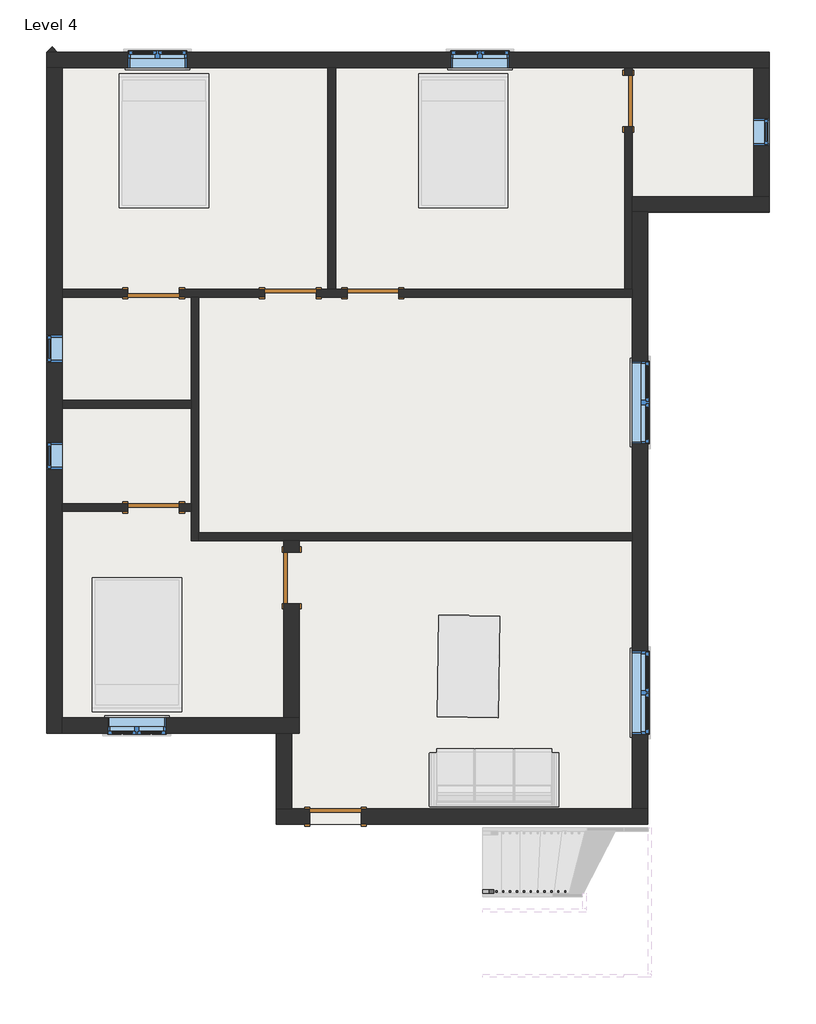
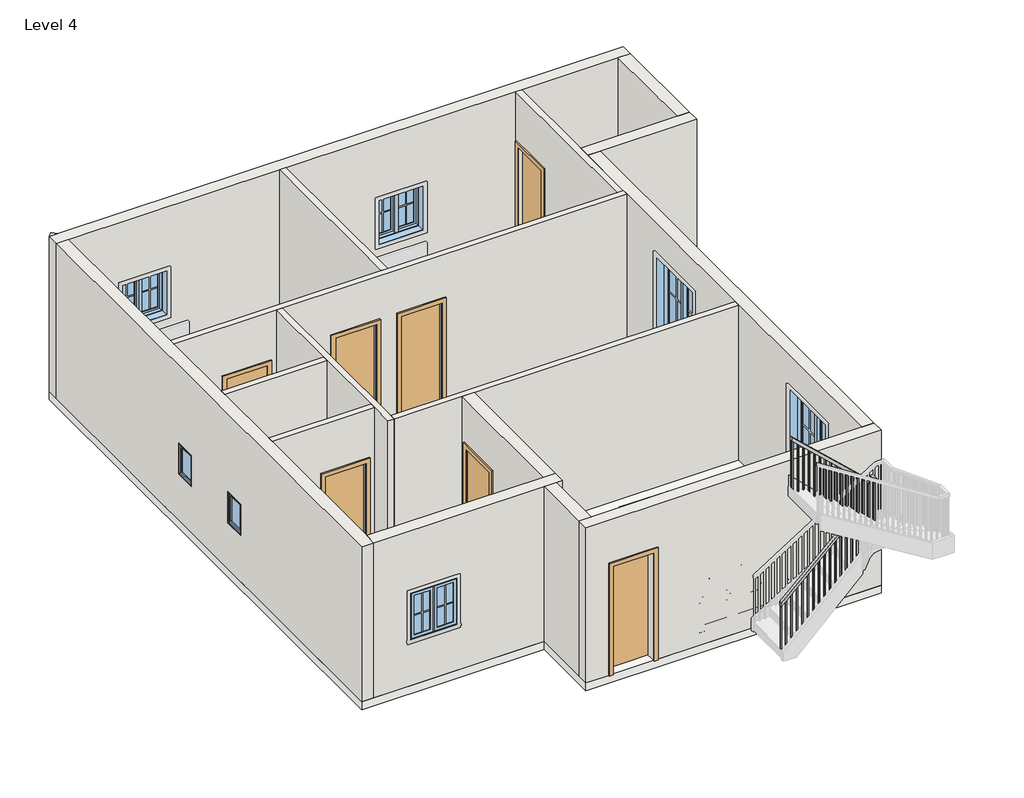
# One storey, part 1 of 2: 17 walls, 8 windows, 7 doors, 1 railing, 1 roof.
"""IFC4 building model written with IfcOpenShell, lengths in millimetres."""

from ifc_helpers import new_model, si_unit, frame, origin, place, context, project, spatial, polyline, outline, extrude, faceted_brep, transform, mapped, element, save
from components import door_f2b275c1, door_d8f5dbb5, door_214872d5, door_78caadf7, door_bb98abfd, window_aa618e30, window_339605e1, window_8377141f

model = new_model("IFC4")

# Units and contexts
model_context = context("Model", 3, world=origin())
ifc_project = project(units=[si_unit("LENGTHUNIT", "METRE", prefix="MILLI")], contexts=[model_context])

# Site, building, storey
site = spatial("IfcSite", under=ifc_project)
building = spatial("IfcBuilding", under=site)
storey = spatial("IfcBuildingStorey", under=building, Name="Level 4", Elevation=6400.8)

# Doors
placement = place(None, origin())
door_shape = door_f2b275c1(model_context)
element("IfcDoor", 1, ObjectType="Single-Flush : 30\" x 80\"", at=placement, inside=storey, context=model_context, shape_type="MappedRepresentation", body=[
    mapped(door_shape, transform((2459.5084916, 7319.9935985, 6400.8), x_axis=(0.0, 1.0, 0.0), y_axis=(-1.0, 0.0, 0.0), z_axis=(0.0, 0.0, 1.0))),
])
element("IfcDoor", 2, ObjectType="Single-Flush : 30\" x 80\"", at=placement, inside=storey, context=model_context, shape_type="MappedRepresentation", body=[
    mapped(door_shape, transform((-4550.8915084, 4481.5435985, 6400.8), x_axis=(1.0, 0.0, 0.0), y_axis=(0.0, 1.0, 0.0), z_axis=(0.0, 0.0, 1.0))),
])
door_2_shape = door_d8f5dbb5(model_context)
element("IfcDoor", 3, ObjectType="Single-Flush : 30\" x 80\"", at=placement, inside=storey, context=model_context, shape_type="MappedRepresentation", body=[
    mapped(door_2_shape, transform((-4550.8915084, 1319.2435985, 6400.8), x_axis=(1.0, 0.0, 0.0), y_axis=(0.0, 1.0, 0.0), z_axis=(0.0, 0.0, 1.0))),
])
door_3_shape = door_214872d5(model_context)
element("IfcDoor", 4, ObjectType="Single-Flush : 30\" x 84\"", at=placement, inside=storey, context=model_context, shape_type="MappedRepresentation", body=[
    mapped(door_3_shape, transform((-2531.5915084, 4481.5435985, 6400.8), x_axis=(1.0, 0.0, 0.0), y_axis=(0.0, 1.0, 0.0), z_axis=(0.0, 0.0, 1.0))),
])
door_4_shape = door_78caadf7(model_context)
element("IfcDoor", 5, ObjectType="Single-Flush : 30\" x 84\"", at=placement, inside=storey, context=model_context, shape_type="MappedRepresentation", body=[
    mapped(door_4_shape, transform((-1312.3915084, 4481.5435985, 6400.8), x_axis=(-1.0, 0.0, 0.0), y_axis=(0.0, -1.0, 0.0), z_axis=(0.0, 0.0, 1.0))),
])
door_5_shape = door_bb98abfd(model_context)
element("IfcDoor", 6, ObjectType="Single-Flush : 30\" x 84\"", at=placement, inside=storey, context=model_context, shape_type="MappedRepresentation", body=[
    mapped(door_5_shape, transform((-2512.5415084, 277.8435985, 6400.8), x_axis=(0.0, 1.0, 0.0), y_axis=(-1.0, 0.0, 0.0), z_axis=(0.0, 0.0, 1.0))),
])
element("IfcDoor", 7, ObjectType="Single-Flush : 30\" x 84\"", at=placement, inside=storey, context=model_context, shape_type="MappedRepresentation", body=[
    mapped(door_5_shape, transform((-1864.8415084, -3246.4064015, 6400.8), x_axis=(1.0, 0.0, 0.0), y_axis=(0.0, 1.0, 0.0), z_axis=(0.0, 0.0, 1.0))),
])

# Railing
element("IfcRailing", 8, ObjectType="Handrail - Rectangular", at=placement, inside=storey, context=model_context, shape_type="SolidModel", body=[
    faceted_brep([(306.9570026, -4325.9064015, 7518.4), (306.9570026, -4325.9064015, 7448.9424448), (306.9570026, -4376.7064015, 7448.9424448), (306.9570026, -4376.7064015, 7518.4), (1758.4886944, -4325.9064015, 8871.8629243), (1809.2886944, -4325.9064015, 8849.773206), (1809.2886944, -4376.7064015, 8849.773206), (1758.4886944, -4376.7064015, 8871.8629243), (1758.4886944, -4325.9064015, 9115.4738258), (1809.2886944, -4325.9064015, 9064.6738258), (1809.2886944, -4376.7064015, 9064.6738258), (1758.4886944, -4376.7064015, 9115.4738258), (1885.4886944, -4325.9064015, 9115.4738258), (1885.4886944, -4325.9064015, 9064.6738258), (1834.6886944, -4376.7064015, 9064.6738258), (1834.6886944, -4376.7064015, 9115.4738258), (1885.4886944, -4452.9064015, 9115.4738258), (1885.4886944, -4484.6424812, 9064.6738258), (1834.6886944, -4484.6424812, 9064.6738258), (1834.6886944, -4452.9064015, 9115.4738258), (1885.4886944, -4579.9064015, 9375.7261742), (1885.4886944, -4630.7064015, 9363.9925523), (1834.6886944, -4630.7064015, 9363.9925523), (1834.6886944, -4579.9064015, 9375.7261742), (1885.4886944, -4579.9064015, 9619.3370757), (1885.4886944, -4630.7064015, 9568.5370757), (1834.6886944, -4630.7064015, 9568.5370757), (1834.6886944, -4579.9064015, 9619.3370757), (1885.4886944, -4706.9064015, 9619.3370757), (1885.4886944, -4706.9064015, 9568.5370757), (1834.6886944, -4656.1064015, 9568.5370757), (1834.6886944, -4656.1064015, 9619.3370757), (1758.4886944, -4706.9064015, 9619.3370757), (1738.4792562, -4706.9064015, 9568.5370757), (1738.4792562, -4656.1064015, 9568.5370757), (1758.4886944, -4656.1064015, 9619.3370757), (306.9570026, -4706.9064015, 10972.8), (306.9570026, -4656.1064015, 10972.8), (306.9570026, -4656.1064015, 10903.3424448), (306.9570026, -4706.9064015, 10903.3424448)], [[[0, 1, 2, 3]], [[1, 0, 4, 5]], [[2, 1, 5, 6]], [[3, 2, 6, 7]], [[0, 3, 7, 4]], [[5, 4, 8, 9]], [[6, 5, 9, 10]], [[7, 6, 10, 11]], [[4, 7, 11, 8]], [[9, 8, 12, 13]], [[10, 9, 13, 14]], [[11, 10, 14, 15]], [[8, 11, 15, 12]], [[13, 12, 16, 17]], [[14, 13, 17, 18]], [[15, 14, 18, 19]], [[12, 15, 19, 16]], [[17, 16, 20, 21]], [[18, 17, 21, 22]], [[19, 18, 22, 23]], [[16, 19, 23, 20]], [[21, 20, 24, 25]], [[22, 21, 25, 26]], [[23, 22, 26, 27]], [[20, 23, 27, 24]], [[25, 24, 28, 29]], [[26, 25, 29, 30]], [[27, 26, 30, 31]], [[24, 27, 31, 28]], [[29, 28, 32, 33]], [[30, 29, 33, 34]], [[31, 30, 34, 35]], [[28, 31, 35, 32]], [[36, 37, 38, 39]], [[33, 32, 36, 39]], [[34, 33, 39, 38]], [[35, 34, 38, 37]], [[32, 35, 37, 36]]]),
    extrude(outline(polyline([(10867.2974865, 345.6136944), (10885.0604254, 326.5636944), (9855.2, 326.5636944), (9855.2, 345.6136944), (10867.2974865, 345.6136944)])), frame((0.0, -4691.0314015, 0.0), z_axis=(0.0, 1.0, 0.0), x_axis=(0.0, 0.0, 1.0)), (0.0, 0.0, 1.0), 19.05),
    extrude(outline(polyline([(10772.5618126, 447.2136944), (10790.3247514, 428.1636944), (9855.2, 428.1636944), (9855.2, 447.2136944), (10772.5618126, 447.2136944)])), frame((0.0, -4691.0314015, 0.0), z_axis=(0.0, 1.0, 0.0), x_axis=(0.0, 0.0, 1.0)), (0.0, 0.0, 1.0), 19.05),
    extrude(outline(polyline([(10677.8261386, 548.8136944), (10695.5890775, 529.7636944), (9855.2, 529.7636944), (9855.2, 548.8136944), (10677.8261386, 548.8136944)])), frame((0.0, -4691.0314015, 0.0), z_axis=(0.0, 1.0, 0.0), x_axis=(0.0, 0.0, 1.0)), (0.0, 0.0, 1.0), 19.05),
    extrude(outline(polyline([(10583.0904646, 650.4136944), (10600.8534035, 631.3636944), (9652.0, 631.3636944), (9652.0, 650.4136944), (10583.0904646, 650.4136944)])), frame((0.0, -4691.0314015, 0.0), z_axis=(0.0, 1.0, 0.0), x_axis=(0.0, 0.0, 1.0)), (0.0, 0.0, 1.0), 19.05),
    extrude(outline(polyline([(10488.3547907, 752.0136944), (10506.1177295, 732.9636944), (9652.0, 732.9636944), (9652.0, 752.0136944), (10488.3547907, 752.0136944)])), frame((0.0, -4691.0314015, 0.0), z_axis=(0.0, 1.0, 0.0), x_axis=(0.0, 0.0, 1.0)), (0.0, 0.0, 1.0), 19.05),
    extrude(outline(polyline([(10393.6191167, 853.6136944), (10411.3820556, 834.5636944), (9652.0, 834.5636944), (9652.0, 853.6136944), (10393.6191167, 853.6136944)])), frame((0.0, -4691.0314015, 0.0), z_axis=(0.0, 1.0, 0.0), x_axis=(0.0, 0.0, 1.0)), (0.0, 0.0, 1.0), 19.05),
    extrude(outline(polyline([(10298.8834427, 955.2136944), (10316.6463816, 936.1636944), (9448.8, 936.1636944), (9448.8, 955.2136944), (10298.8834427, 955.2136944)])), frame((0.0, -4691.0314015, 0.0), z_axis=(0.0, 1.0, 0.0), x_axis=(0.0, 0.0, 1.0)), (0.0, 0.0, 1.0), 19.05),
    extrude(outline(polyline([(10204.1477688, 1056.8136944), (10221.9107076, 1037.7636944), (9448.8, 1037.7636944), (9448.8, 1056.8136944), (10204.1477688, 1056.8136944)])), frame((0.0, -4691.0314015, 0.0), z_axis=(0.0, 1.0, 0.0), x_axis=(0.0, 0.0, 1.0)), (0.0, 0.0, 1.0), 19.05),
    extrude(outline(polyline([(10109.4120948, 1158.4136944), (10127.1750337, 1139.3636944), (9245.6, 1139.3636944), (9245.6, 1158.4136944), (10109.4120948, 1158.4136944)])), frame((0.0, -4691.0314015, 0.0), z_axis=(0.0, 1.0, 0.0), x_axis=(0.0, 0.0, 1.0)), (0.0, 0.0, 1.0), 19.05),
    extrude(outline(polyline([(10014.6764208, 1260.0136944), (10032.4393597, 1240.9636944), (9245.6, 1240.9636944), (9245.6, 1260.0136944), (10014.6764208, 1260.0136944)])), frame((0.0, -4691.0314015, 0.0), z_axis=(0.0, 1.0, 0.0), x_axis=(0.0, 0.0, 1.0)), (0.0, 0.0, 1.0), 19.05),
    extrude(outline(polyline([(9919.9407469, 1361.6136944), (9937.7036857, 1342.5636944), (9245.6, 1342.5636944), (9245.6, 1361.6136944), (9919.9407469, 1361.6136944)])), frame((0.0, -4691.0314015, 0.0), z_axis=(0.0, 1.0, 0.0), x_axis=(0.0, 0.0, 1.0)), (0.0, 0.0, 1.0), 19.05),
    extrude(outline(polyline([(9825.2050729, 1463.2136944), (9842.9680118, 1444.1636944), (9042.4, 1444.1636944), (9042.4, 1463.2136944), (9825.2050729, 1463.2136944)])), frame((0.0, -4691.0314015, 0.0), z_axis=(0.0, 1.0, 0.0), x_axis=(0.0, 0.0, 1.0)), (0.0, 0.0, 1.0), 19.05),
    extrude(outline(polyline([(9730.4693989, 1564.8136944), (9748.2323378, 1545.7636944), (9042.4, 1545.7636944), (9042.4, 1564.8136944), (9730.4693989, 1564.8136944)])), frame((0.0, -4691.0314015, 0.0), z_axis=(0.0, 1.0, 0.0), x_axis=(0.0, 0.0, 1.0)), (0.0, 0.0, 1.0), 19.05),
    extrude(outline(polyline([(9635.733725, 1666.4136944), (9653.4966638, 1647.3636944), (8839.2, 1647.3636944), (8839.2, 1666.4136944), (9635.733725, 1666.4136944)])), frame((0.0, -4691.0314015, 0.0), z_axis=(0.0, 1.0, 0.0), x_axis=(0.0, 0.0, 1.0)), (0.0, 0.0, 1.0), 19.05),
    extrude(outline(polyline([(9540.998051, 1768.0136944), (9558.7609899, 1748.9636944), (8839.2, 1748.9636944), (8839.2, 1768.0136944), (9540.998051, 1768.0136944)])), frame((0.0, -4691.0314015, 0.0), z_axis=(0.0, 1.0, 0.0), x_axis=(0.0, 0.0, 1.0)), (0.0, 0.0, 1.0), 19.05),
    extrude(outline(polyline([(1850.5636944, -4646.5814015), (1869.6136944, -4646.5814015), (1869.6136944, -4665.6314015), (1850.5636944, -4665.6314015), (1850.5636944, -4646.5814015)])), frame((0.0, 0.0, 8432.8), z_axis=(0.0, 0.0, 1.0), x_axis=(1.0, 0.0, 0.0)), (0.0, 0.0, 1.0), 1135.7370757),
    extrude(outline(polyline([(-4564.0314015, 9227.3600694), (-4544.9814015, 9188.3222172), (-4544.9814015, 8229.6), (-4564.0314015, 8229.6), (-4564.0314015, 9227.3600694)])), frame((1850.5636944, 0.0, 0.0), z_axis=(1.0, 0.0, 0.0), x_axis=(0.0, 1.0, 0.0)), (0.0, 0.0, 1.0), 19.05),
    extrude(outline(polyline([(-4462.4314015, 9019.1581907), (-4443.3814015, 8980.1203385), (-4443.3814015, 8026.4), (-4462.4314015, 8026.4), (-4462.4314015, 9019.1581907)])), frame((1850.5636944, 0.0, 0.0), z_axis=(1.0, 0.0, 0.0), x_axis=(0.0, 1.0, 0.0)), (0.0, 0.0, 1.0), 19.05),
    extrude(outline(polyline([(1821.4320026, -4360.8314015), (1821.4320026, -4341.7814015), (1840.4820026, -4341.7814015), (1840.4820026, -4360.8314015), (1821.4320026, -4360.8314015)])), frame((0.0, 0.0, 7823.2), z_axis=(0.0, 0.0, 1.0), x_axis=(1.0, 0.0, 0.0)), (0.0, 0.0, 1.0), 1241.4738258),
    extrude(outline(polyline([(8784.1233497, 1738.8820026), (8766.3604108, 1719.8320026), (7620.0, 1719.8320026), (7620.0, 1738.8820026), (8784.1233497, 1738.8820026)])), frame((0.0, -4360.8314015, 0.0), z_axis=(0.0, 1.0, 0.0), x_axis=(0.0, 0.0, 1.0)), (0.0, 0.0, 1.0), 19.05),
    extrude(outline(polyline([(8689.3876757, 1637.2820026), (8671.6247369, 1618.2320026), (7620.0, 1618.2320026), (7620.0, 1637.2820026), (8689.3876757, 1637.2820026)])), frame((0.0, -4360.8314015, 0.0), z_axis=(0.0, 1.0, 0.0), x_axis=(0.0, 0.0, 1.0)), (0.0, 0.0, 1.0), 19.05),
    extrude(outline(polyline([(8594.6520018, 1535.6820026), (8576.8890629, 1516.6320026), (7416.8, 1516.6320026), (7416.8, 1535.6820026), (8594.6520018, 1535.6820026)])), frame((0.0, -4360.8314015, 0.0), z_axis=(0.0, 1.0, 0.0), x_axis=(0.0, 0.0, 1.0)), (0.0, 0.0, 1.0), 19.05),
    extrude(outline(polyline([(8499.9163278, 1434.0820026), (8482.1533889, 1415.0320026), (7416.8, 1415.0320026), (7416.8, 1434.0820026), (8499.9163278, 1434.0820026)])), frame((0.0, -4360.8314015, 0.0), z_axis=(0.0, 1.0, 0.0), x_axis=(0.0, 0.0, 1.0)), (0.0, 0.0, 1.0), 19.05),
    extrude(outline(polyline([(8405.1806538, 1332.4820026), (8387.417715, 1313.4320026), (7213.6, 1313.4320026), (7213.6, 1332.4820026), (8405.1806538, 1332.4820026)])), frame((0.0, -4360.8314015, 0.0), z_axis=(0.0, 1.0, 0.0), x_axis=(0.0, 0.0, 1.0)), (0.0, 0.0, 1.0), 19.05),
    extrude(outline(polyline([(8310.4449799, 1230.8820026), (8292.682041, 1211.8320026), (7213.6, 1211.8320026), (7213.6, 1230.8820026), (8310.4449799, 1230.8820026)])), frame((0.0, -4360.8314015, 0.0), z_axis=(0.0, 1.0, 0.0), x_axis=(0.0, 0.0, 1.0)), (0.0, 0.0, 1.0), 19.05),
    extrude(outline(polyline([(8215.7093059, 1129.2820026), (8197.946367, 1110.2320026), (7010.4, 1110.2320026), (7010.4, 1129.2820026), (8215.7093059, 1129.2820026)])), frame((0.0, -4360.8314015, 0.0), z_axis=(0.0, 1.0, 0.0), x_axis=(0.0, 0.0, 1.0)), (0.0, 0.0, 1.0), 19.05),
    extrude(outline(polyline([(8120.9736319, 1027.6820026), (8103.2106931, 1008.6320026), (7010.4, 1008.6320026), (7010.4, 1027.6820026), (8120.9736319, 1027.6820026)])), frame((0.0, -4360.8314015, 0.0), z_axis=(0.0, 1.0, 0.0), x_axis=(0.0, 0.0, 1.0)), (0.0, 0.0, 1.0), 19.05),
    extrude(outline(polyline([(8026.237958, 926.0820026), (8008.4750191, 907.0320026), (7010.4, 907.0320026), (7010.4, 926.0820026), (8026.237958, 926.0820026)])), frame((0.0, -4360.8314015, 0.0), z_axis=(0.0, 1.0, 0.0), x_axis=(0.0, 0.0, 1.0)), (0.0, 0.0, 1.0), 19.05),
    extrude(outline(polyline([(7931.502284, 824.4820026), (7913.7393451, 805.4320026), (6807.2, 805.4320026), (6807.2, 824.4820026), (7931.502284, 824.4820026)])), frame((0.0, -4360.8314015, 0.0), z_axis=(0.0, 1.0, 0.0), x_axis=(0.0, 0.0, 1.0)), (0.0, 0.0, 1.0), 19.05),
    extrude(outline(polyline([(7836.7666101, 722.8820026), (7819.0036712, 703.8320026), (6807.2, 703.8320026), (6807.2, 722.8820026), (7836.7666101, 722.8820026)])), frame((0.0, -4360.8314015, 0.0), z_axis=(0.0, 1.0, 0.0), x_axis=(0.0, 0.0, 1.0)), (0.0, 0.0, 1.0), 19.05),
    extrude(outline(polyline([(7742.0309361, 621.2820026), (7724.2679972, 602.2320026), (6807.2, 602.2320026), (6807.2, 621.2820026), (7742.0309361, 621.2820026)])), frame((0.0, -4360.8314015, 0.0), z_axis=(0.0, 1.0, 0.0), x_axis=(0.0, 0.0, 1.0)), (0.0, 0.0, 1.0), 19.05),
    extrude(outline(polyline([(7647.2952621, 519.6820026), (7629.5323233, 500.6320026), (6604.0, 500.6320026), (6604.0, 519.6820026), (7647.2952621, 519.6820026)])), frame((0.0, -4360.8314015, 0.0), z_axis=(0.0, 1.0, 0.0), x_axis=(0.0, 0.0, 1.0)), (0.0, 0.0, 1.0), 19.05),
    extrude(outline(polyline([(7552.5595882, 418.0820026), (7534.7966493, 399.0320026), (6604.0, 399.0320026), (6604.0, 418.0820026), (7552.5595882, 418.0820026)])), frame((0.0, -4360.8314015, 0.0), z_axis=(0.0, 1.0, 0.0), x_axis=(0.0, 0.0, 1.0)), (0.0, 0.0, 1.0), 19.05),
    extrude(outline(polyline([(1850.5636944, -4671.9814015), (1869.6136944, -4671.9814015), (1869.6136944, -4691.0314015), (1850.5636944, -4691.0314015), (1850.5636944, -4671.9814015)])), frame((0.0, 0.0, 8636.0), z_axis=(0.0, 0.0, 1.0), x_axis=(1.0, 0.0, 0.0)), (0.0, 0.0, 1.0), 932.5370757),
    extrude(outline(polyline([(1850.5636944, -4360.8314015), (1850.5636944, -4341.7814015), (1869.6136944, -4341.7814015), (1869.6136944, -4360.8314015), (1850.5636944, -4360.8314015)])), frame((0.0, 0.0, 7823.2), z_axis=(0.0, 0.0, 1.0), x_axis=(1.0, 0.0, 0.0)), (0.0, 0.0, 1.0), 1241.4738258),
    extrude(outline(polyline([(10885.5795059, 326.0070026), (10903.3424448, 306.9570026), (9855.2, 306.9570026), (9855.2, 326.0070026), (10885.5795059, 326.0070026)])), frame((0.0, -4691.0314015, 0.0), z_axis=(0.0, 1.0, 0.0), x_axis=(0.0, 0.0, 1.0)), (0.0, 0.0, 1.0), 19.05),
    extrude(outline(polyline([(7466.7053836, 326.0070026), (7448.9424448, 306.9570026), (6604.0, 306.9570026), (6604.0, 326.0070026), (7466.7053836, 326.0070026)])), frame((0.0, -4360.8314015, 0.0), z_axis=(0.0, 1.0, 0.0), x_axis=(0.0, 0.0, 1.0)), (0.0, 0.0, 1.0), 19.05),
])

# Roof
element("IfcRoof", 9, ObjectType="Generic - 12\"", at=placement, inside=storey, context=model_context, shape_type="SweptSolid", body=[
    extrude(outline(polyline([(-6132.0415084, 8043.8940003), (4535.9584916, 8043.8940003), (4535.9584916, 5681.6935985), (2745.2584916, 5681.6935985), (2745.2584916, -3360.7064015), (-2741.1415084, -3360.7064015), (-2741.1415084, -2014.5064015), (-6132.0415084, -2014.5064015), (-6132.0415084, 8043.8940003)])), frame((0.0, 0.0, 6248.4), z_axis=(0.0, 0.0, 1.0), x_axis=(1.0, 0.0, 0.0)), (0.0, 0.0, 1.0), 152.4),
])

# Walls
element("IfcWall", 10, ObjectType="WALL4.5\"", at=placement, inside=storey, context=model_context, shape_type="SweptSolid", body=[
    extrude(outline(polyline([(-1979.1415084, 4538.6935985), (-1979.1415084, 7815.2935985), (-1864.8415084, 7815.2935985), (-1864.8415084, 4538.6935985), (-1979.1415084, 4538.6935985)])), frame((0.0, 0.0, 6400.8), z_axis=(0.0, 0.0, 1.0), x_axis=(1.0, 0.0, 0.0)), (0.0, 0.0, 1.0), 3048.0),
])
element("IfcWall", 11, ObjectType="WALL4.5\"", at=placement, inside=storey, context=model_context, shape_type="Brep", body=[
    faceted_brep([(-2150.5915084, 4424.3935985, 6400.8), (-1693.3915084, 4424.3935985, 6400.8), (-1693.3915084, 4424.3935985, 8534.4), (-931.3915084, 4424.3935985, 8534.4), (-931.3915084, 4424.3935985, 6400.8), (2516.6584916, 4424.3935985, 6400.8), (2516.6584916, 4424.3935985, 9448.8), (-3884.1415084, 4424.3935985, 9448.8), (-3998.4415084, 4424.3935985, 9448.8), (-5903.4415084, 4424.3935985, 9448.8), (-5903.4415084, 4424.3935985, 6400.8), (-4931.8915084, 4424.3935985, 6400.8), (-4931.8915084, 4424.3935985, 8432.8), (-4169.8915084, 4424.3935985, 8432.8), (-4169.8915084, 4424.3935985, 6400.8), (-3998.4415084, 4424.3935985, 6400.8), (-3884.1415084, 4424.3935985, 6400.8), (-2912.5915084, 4424.3935985, 6400.8), (-2912.5915084, 4424.3935985, 8534.4), (-2150.5915084, 4424.3935985, 8534.4), (-1693.3915084, 4538.6935985, 8534.4), (-1693.3915084, 4538.6935985, 6400.8), (-1864.8415084, 4538.6935985, 6400.8), (-1979.1415084, 4538.6935985, 6400.8), (-2150.5915084, 4538.6935985, 6400.8), (-2150.5915084, 4538.6935985, 8534.4), (-2912.5915084, 4538.6935985, 8534.4), (-2912.5915084, 4538.6935985, 6400.8), (-4169.8915084, 4538.6935985, 6400.8), (-4169.8915084, 4538.6935985, 8432.8), (-4931.8915084, 4538.6935985, 8432.8), (-4931.8915084, 4538.6935985, 6400.8), (-5903.4415084, 4538.6935985, 6400.8), (-5903.4415084, 4538.6935985, 9448.8), (-1979.1415084, 4538.6935985, 9448.8), (-1864.8415084, 4538.6935985, 9448.8), (2402.3584916, 4538.6935985, 9448.8), (2516.6584916, 4538.6935985, 9448.8), (2516.6584916, 4538.6935985, 6400.8), (2402.3584916, 4538.6935985, 6400.8), (-931.3915084, 4538.6935985, 6400.8), (-931.3915084, 4538.6935985, 8534.4)], [[[0, 1, 2, 3, 4, 5, 6, 7, 8, 9, 10, 11, 12, 13, 14, 15, 16, 17, 18, 19]], [[20, 21, 22, 23, 24, 25, 26, 27, 28, 29, 30, 31, 32, 33, 34, 35, 36, 37, 38, 39, 40, 41]], [[11, 10, 32, 31]], [[17, 16, 15, 14, 28, 27]], [[40, 39, 38, 5, 4]], [[24, 23, 22, 21, 1, 0]], [[10, 9, 33, 32]], [[6, 5, 38, 37]], [[29, 28, 14, 13]], [[30, 29, 13, 12]], [[31, 30, 12, 11]], [[25, 24, 0, 19]], [[26, 25, 19, 18]], [[27, 26, 18, 17]], [[2, 1, 21, 20]], [[3, 2, 20, 41]], [[4, 3, 41, 40]], [[9, 8, 7, 6, 37, 36, 35, 34, 33]]]),
])
element("IfcWall", 12, ObjectType="WALL4.5\"", at=placement, inside=storey, context=model_context, shape_type="Brep", body=[
    faceted_brep([(2516.6584916, 7700.9935985, 8432.8), (2516.6584916, 7700.9935985, 6400.8), (2516.6584916, 7815.2935985, 6400.8), (2516.6584916, 7815.2935985, 9448.8), (2516.6584916, 5910.2935985, 9448.8), (2516.6584916, 5681.6935985, 9448.8), (2516.6584916, 4538.6935985, 9448.8), (2516.6584916, 4538.6935985, 6400.8), (2516.6584916, 5681.6935985, 6400.8), (2516.6584916, 5910.2935985, 6400.8), (2516.6584916, 6938.9935985, 6400.8), (2516.6584916, 6938.9935985, 8432.8), (2402.3584916, 7815.2935985, 6400.8), (2402.3584916, 7700.9935985, 6400.8), (2402.3584916, 7700.9935985, 8432.8), (2402.3584916, 6938.9935985, 8432.8), (2402.3584916, 6938.9935985, 6400.8), (2402.3584916, 4538.6935985, 6400.8), (2402.3584916, 4538.6935985, 9448.8), (2402.3584916, 7815.2935985, 9448.8)], [[[0, 1, 2, 3, 4, 5, 6, 7, 8, 9, 10, 11]], [[12, 13, 14, 15, 16, 17, 18, 19]], [[2, 1, 13, 12]], [[10, 9, 8, 7, 17, 16]], [[7, 6, 18, 17]], [[3, 2, 12, 19]], [[14, 13, 1, 0]], [[15, 14, 0, 11]], [[16, 15, 11, 10]], [[6, 5, 4, 3, 19, 18]]]),
])
element("IfcWall", 13, ObjectType="WALL4.5\"", at=placement, inside=storey, context=model_context, shape_type="Brep", body=[
    faceted_brep([(-3998.4415084, 4424.3935985, 6400.8), (-3998.4415084, 2900.3935985, 6400.8), (-3998.4415084, 2786.0935985, 6400.8), (-3998.4415084, 1376.3935985, 6400.8), (-3998.4415084, 1262.0935985, 6400.8), (-3998.4415084, 830.2935985, 6400.8), (-3998.4415084, 830.2935985, 9448.8), (-3998.4415084, 1262.0935985, 9448.8), (-3998.4415084, 1376.3935985, 9448.8), (-3998.4415084, 2786.0935985, 9448.8), (-3998.4415084, 2900.3935985, 9448.8), (-3998.4415084, 4424.3935985, 9448.8), (-3884.1415084, 4424.3935985, 6400.8), (-3884.1415084, 4424.3935985, 9448.8), (-3884.1415084, 944.5935985, 9448.8), (-3884.1415084, 830.2935985, 9448.8), (-3884.1415084, 830.2935985, 6400.8), (-3884.1415084, 944.5935985, 6400.8)], [[[0, 1, 2, 3, 4, 5, 6, 7, 8, 9, 10, 11]], [[12, 13, 14, 15, 16, 17]], [[5, 4, 3, 2, 1, 0, 12, 17, 16]], [[0, 11, 13, 12]], [[6, 5, 16, 15]], [[11, 10, 9, 8, 7, 6, 15, 14, 13]]]),
])
element("IfcWall", 14, ObjectType="WALL4.5\"", at=placement, inside=storey, context=model_context, shape_type="Brep", body=[
    faceted_brep([(-3884.1415084, 830.2935985, 6400.8), (-2626.8415084, 830.2935985, 6400.8), (-2398.2415084, 830.2935985, 6400.8), (2516.6584916, 830.2935985, 6400.8), (2516.6584916, 830.2935985, 9448.8), (-2398.2415084, 830.2935985, 9448.8), (-2626.8415084, 830.2935985, 9448.8), (-3884.1415084, 830.2935985, 9448.8), (-3884.1415084, 944.5935985, 6400.8), (-3884.1415084, 944.5935985, 9448.8), (2516.6584916, 944.5935985, 9448.8), (2516.6584916, 944.5935985, 6400.8)], [[[0, 1, 2, 3, 4, 5, 6, 7]], [[8, 9, 10, 11]], [[3, 2, 1, 0, 8, 11]], [[0, 7, 9, 8]], [[4, 3, 11, 10]], [[7, 6, 5, 4, 10, 9]]]),
])
element("IfcWall", 15, ObjectType="WALL4.5\"", at=placement, inside=storey, context=model_context, shape_type="SweptSolid", body=[
    extrude(outline(polyline([(-3998.4415084, 2786.0935985), (-5903.4415084, 2786.0935985), (-5903.4415084, 2900.3935985), (-3998.4415084, 2900.3935985), (-3998.4415084, 2786.0935985)])), frame((0.0, 0.0, 6400.8), z_axis=(0.0, 0.0, 1.0), x_axis=(1.0, 0.0, 0.0)), (0.0, 0.0, 1.0), 3048.0),
])
element("IfcWall", 16, ObjectType="WALL4.5\"", at=placement, inside=storey, context=model_context, shape_type="SweptSolid", body=[
    extrude(outline(polyline([(8432.8, -4169.8915084), (6400.8, -4169.8915084), (6400.8, -3998.4415084), (9448.8, -3998.4415084), (9448.8, -5903.4415084), (6400.8, -5903.4415084), (6400.8, -4931.8915084), (8432.8, -4931.8915084), (8432.8, -4169.8915084)])), frame((0.0, 1262.0935985, 0.0), z_axis=(0.0, 1.0, 0.0), x_axis=(0.0, 0.0, 1.0)), (0.0, 0.0, 1.0), 114.3),
])
element("IfcWall", 17, ObjectType="WALL4.5\"", at=placement, inside=storey, context=model_context, shape_type="SweptSolid", body=[
    extrude(outline(polyline([(-6051.2188015, 8124.7159036), (-5970.3964964, 8043.8935985), (-6132.0411066, 8043.8935985), (-6051.2188015, 8124.7159036)])), frame((0.0, 0.0, 6400.8), z_axis=(0.0, 0.0, 1.0), x_axis=(1.0, 0.0, 0.0)), (0.0, 0.0, 1.0), 3048.0),
])
element("IfcWall", 18, ObjectType="WALL9\"", at=placement, inside=storey, context=model_context, shape_type="Brep", body=[
    faceted_brep([(-6132.0415084, 7815.2935985, 6400.8), (-5903.4415084, 7815.2935985, 6400.8), (-1979.1415084, 7815.2935985, 6400.8), (-1864.8415084, 7815.2935985, 6400.8), (2402.3584916, 7815.2935985, 6400.8), (2516.6584916, 7815.2935985, 6400.8), (4307.3584916, 7815.2935985, 6400.8), (4535.9584916, 7815.2935985, 6400.8), (4535.9584916, 7815.2935985, 9448.8), (4307.3584916, 7815.2935985, 9448.8), (2516.6584916, 7815.2935985, 9448.8), (2402.3584916, 7815.2935985, 9448.8), (-1864.8415084, 7815.2935985, 9448.8), (-1979.1415084, 7815.2935985, 9448.8), (-5903.4415084, 7815.2935985, 9448.8), (-6132.0415084, 7815.2935985, 9448.8), (-4061.9415084, 7815.2935985, 8229.6), (-4061.9415084, 7815.2935985, 7315.2), (-4925.5415084, 7815.2935985, 7315.2), (-4925.5415084, 7815.2935985, 8229.6), (700.5584916, 7815.2935985, 8229.6), (700.5584916, 7815.2935985, 7315.2), (-163.0415084, 7815.2935985, 7315.2), (-163.0415084, 7815.2935985, 8229.6), (-6132.0415084, 8043.8935985, 6400.8), (-6132.0415084, 8043.8935985, 9448.8), (-5970.3964964, 8043.8935985, 9448.8), (4535.9584916, 8043.8935985, 9448.8), (4535.9584916, 8043.8935985, 6400.8), (-5970.3964964, 8043.8935985, 6400.8), (-4061.9415084, 8043.8935985, 8229.6), (-4925.5415084, 8043.8935985, 8229.6), (-4925.5415084, 8043.8935985, 7315.2), (-4061.9415084, 8043.8935985, 7315.2), (700.5584916, 8043.8935985, 8229.6), (-163.0415084, 8043.8935985, 8229.6), (-163.0415084, 8043.8935985, 7315.2), (700.5584916, 8043.8935985, 7315.2)], [[[0, 1, 2, 3, 4, 5, 6, 7, 8, 9, 10, 11, 12, 13, 14, 15], [16, 17, 18, 19], [20, 21, 22, 23]], [[24, 25, 26, 27, 28, 29], [30, 31, 32, 33], [34, 35, 36, 37]], [[7, 6, 5, 4, 3, 2, 1, 0, 24, 29, 28]], [[0, 15, 25, 24]], [[8, 7, 28, 27]], [[17, 16, 30, 33]], [[18, 17, 33, 32]], [[19, 18, 32, 31]], [[16, 19, 31, 30]], [[21, 20, 34, 37]], [[22, 21, 37, 36]], [[23, 22, 36, 35]], [[20, 23, 35, 34]], [[15, 14, 13, 12, 11, 10, 9, 8, 27, 26, 25]]]),
])
element("IfcWall", 19, ObjectType="WALL9\"", at=placement, inside=storey, context=model_context, shape_type="Brep", body=[
    faceted_brep([(-6132.0415084, 7815.2935985, 6400.8), (-6132.0415084, -2014.5064015, 6400.8), (-6132.0415084, -2014.5064015, 9448.8), (-6132.0415084, 7815.2935985, 9448.8), (-6132.0415084, 3865.5935985, 7924.8), (-6132.0415084, 3459.1935985, 7924.8), (-6132.0415084, 3459.1935985, 7315.2), (-6132.0415084, 3865.5935985, 7315.2), (-6132.0415084, 2284.4435985, 7924.8), (-6132.0415084, 1878.0435985, 7924.8), (-6132.0415084, 1878.0435985, 7315.2), (-6132.0415084, 2284.4435985, 7315.2), (-5903.4415084, 7815.2935985, 6400.8), (-5903.4415084, 7815.2935985, 9448.8), (-5903.4415084, 4538.6935985, 9448.8), (-5903.4415084, 4424.3935985, 9448.8), (-5903.4415084, 2900.3935985, 9448.8), (-5903.4415084, 2786.0935985, 9448.8), (-5903.4415084, 1376.3935985, 9448.8), (-5903.4415084, 1262.0935985, 9448.8), (-5903.4415084, -1785.9064015, 9448.8), (-5903.4415084, -2014.5064015, 9448.8), (-5903.4415084, -2014.5064015, 6400.8), (-5903.4415084, -1785.9064015, 6400.8), (-5903.4415084, 1262.0935985, 6400.8), (-5903.4415084, 1376.3935985, 6400.8), (-5903.4415084, 2786.0935985, 6400.8), (-5903.4415084, 2900.3935985, 6400.8), (-5903.4415084, 4424.3935985, 6400.8), (-5903.4415084, 4538.6935985, 6400.8), (-5903.4415084, 3865.5935985, 7924.8), (-5903.4415084, 3865.5935985, 7315.2), (-5903.4415084, 3459.1935985, 7315.2), (-5903.4415084, 3459.1935985, 7924.8), (-5903.4415084, 2284.4435985, 7924.8), (-5903.4415084, 2284.4435985, 7315.2), (-5903.4415084, 1878.0435985, 7315.2), (-5903.4415084, 1878.0435985, 7924.8)], [[[0, 1, 2, 3], [4, 5, 6, 7], [8, 9, 10, 11]], [[12, 13, 14, 15, 16, 17, 18, 19, 20, 21, 22, 23, 24, 25, 26, 27, 28, 29], [30, 31, 32, 33], [34, 35, 36, 37]], [[1, 0, 12, 29, 28, 27, 26, 25, 24, 23, 22]], [[0, 3, 13, 12]], [[2, 1, 22, 21]], [[31, 30, 4, 7]], [[32, 31, 7, 6]], [[33, 32, 6, 5]], [[30, 33, 5, 4]], [[35, 34, 8, 11]], [[36, 35, 11, 10]], [[37, 36, 10, 9]], [[34, 37, 9, 8]], [[3, 2, 21, 20, 19, 18, 17, 16, 15, 14, 13]]]),
])
element("IfcWall", 20, ObjectType="WALL9\"", at=placement, inside=storey, context=model_context, shape_type="Brep", body=[
    faceted_brep([(-5903.4415084, -2014.5064015, 6400.8), (-2741.1415084, -2014.5064015, 6400.8), (-2512.5415084, -2014.5064015, 6400.8), (-2398.2415084, -2014.5064015, 6400.8), (-2398.2415084, -2014.5064015, 9448.8), (-2512.5415084, -2014.5064015, 9448.8), (-2741.1415084, -2014.5064015, 9448.8), (-5903.4415084, -2014.5064015, 9448.8), (-5230.3415084, -2014.5064015, 8229.6), (-4366.7415084, -2014.5064015, 8229.6), (-4366.7415084, -2014.5064015, 7315.2), (-5230.3415084, -2014.5064015, 7315.2), (-5903.4415084, -1785.9064015, 6400.8), (-5903.4415084, -1785.9064015, 9448.8), (-2626.8415084, -1785.9064015, 9448.8), (-2398.2415084, -1785.9064015, 9448.8), (-2398.2415084, -1785.9064015, 6400.8), (-2626.8415084, -1785.9064015, 6400.8), (-5230.3415084, -1785.9064015, 8229.6), (-5230.3415084, -1785.9064015, 7315.2), (-4366.7415084, -1785.9064015, 7315.2), (-4366.7415084, -1785.9064015, 8229.6)], [[[0, 1, 2, 3, 4, 5, 6, 7], [8, 9, 10, 11]], [[12, 13, 14, 15, 16, 17], [18, 19, 20, 21]], [[3, 2, 1, 0, 12, 17, 16]], [[0, 7, 13, 12]], [[4, 3, 16, 15]], [[19, 18, 8, 11]], [[20, 19, 11, 10]], [[21, 20, 10, 9]], [[18, 21, 9, 8]], [[7, 6, 5, 4, 15, 14, 13]]]),
])
element("IfcWall", 21, ObjectType="WALL9\"", at=placement, inside=storey, context=model_context, shape_type="SweptSolid", body=[
    extrude(outline(polyline([(830.2935985, 6400.8), (658.8435985, 6400.8), (658.8435985, 8534.4), (-103.1564015, 8534.4), (-103.1564015, 6400.8), (-1785.9064015, 6400.8), (-1785.9064015, 9448.8), (830.2935985, 9448.8), (830.2935985, 6400.8)])), frame((-2626.8415084, 0.0, 0.0), z_axis=(1.0, 0.0, 0.0), x_axis=(0.0, 1.0, 0.0)), (0.0, 0.0, 1.0), 228.6),
])
element("IfcWall", 22, ObjectType="WALL9\"", at=placement, inside=storey, context=model_context, shape_type="Brep", body=[
    faceted_brep([(2745.2584916, -3132.1064015, 6400.8), (2516.6584916, -3132.1064015, 6400.8), (-1483.8415084, -3132.1064015, 6400.8), (-1483.8415084, -3132.1064015, 8534.4), (-2245.8415084, -3132.1064015, 8534.4), (-2245.8415084, -3132.1064015, 6400.8), (-2512.5415084, -3132.1064015, 6400.8), (-2741.1415084, -3132.1064015, 6400.8), (-2741.1415084, -3132.1064015, 9448.8), (-2512.5415084, -3132.1064015, 9448.8), (2516.6584916, -3132.1064015, 9448.8), (2745.2584916, -3132.1064015, 9448.8), (-1483.8415084, -3360.7064015, 8534.4), (-1483.8415084, -3360.7064015, 6400.8), (2745.2584916, -3360.7064015, 6400.8), (2745.2584916, -3360.7064015, 9448.8), (-2741.1415084, -3360.7064015, 9448.8), (-2741.1415084, -3360.7064015, 6400.8), (-2245.8415084, -3360.7064015, 6400.8), (-2245.8415084, -3360.7064015, 8534.4)], [[[0, 1, 2, 3, 4, 5, 6, 7, 8, 9, 10, 11]], [[12, 13, 14, 15, 16, 17, 18, 19]], [[18, 17, 7, 6, 5]], [[14, 13, 2, 1, 0]], [[8, 7, 17, 16]], [[0, 11, 15, 14]], [[3, 2, 13, 12]], [[4, 3, 12, 19]], [[5, 4, 19, 18]], [[11, 10, 9, 8, 16, 15]]]),
])
element("IfcWall", 23, ObjectType="WALL9\"", at=placement, inside=storey, context=model_context, shape_type="SweptSolid", body=[
    extrude(outline(polyline([(-2512.5415084, -2014.5064015), (-2512.5415084, -3132.1064015), (-2741.1415084, -3132.1064015), (-2741.1415084, -2014.5064015), (-2512.5415084, -2014.5064015)])), frame((0.0, 0.0, 6400.8), z_axis=(0.0, 0.0, 1.0), x_axis=(1.0, 0.0, 0.0)), (0.0, 0.0, 1.0), 3048.0),
])
element("IfcWall", 24, ObjectType="WALL9\"", at=placement, inside=storey, context=model_context, shape_type="Brep", body=[
    faceted_brep([(4535.9584916, 5910.2935985, 6400.8), (4307.3584916, 5910.2935985, 6400.8), (2516.6584916, 5910.2935985, 6400.8), (2516.6584916, 5910.2935985, 9448.8), (4307.3584916, 5910.2935985, 9448.8), (4535.9584916, 5910.2935985, 9448.8), (4535.9584916, 5681.6935985, 6400.8), (4535.9584916, 5681.6935985, 9448.8), (2745.2584916, 5681.6935985, 9448.8), (2516.6584916, 5681.6935985, 9448.8), (2516.6584916, 5681.6935985, 6400.8), (2745.2584916, 5681.6935985, 6400.8)], [[[0, 1, 2, 3, 4, 5]], [[6, 7, 8, 9, 10, 11]], [[2, 1, 0, 6, 11, 10]], [[3, 2, 10, 9]], [[0, 5, 7, 6]], [[5, 4, 3, 9, 8, 7]]]),
])
element("IfcWall", 25, ObjectType="WALL9\"", at=placement, inside=storey, context=model_context, shape_type="Brep", body=[
    faceted_brep([(2516.6584916, 5681.6935985, 6400.8), (2516.6584916, 944.5935985, 6400.8), (2516.6584916, 830.2935985, 6400.8), (2516.6584916, -3132.1064015, 6400.8), (2516.6584916, -3132.1064015, 9448.8), (2516.6584916, 830.2935985, 9448.8), (2516.6584916, 944.5935985, 9448.8), (2516.6584916, 5681.6935985, 9448.8), (2516.6584916, -2027.2064015, 8839.2), (2516.6584916, -2027.2064015, 7315.2), (2516.6584916, -808.0064015, 7315.2), (2516.6584916, -808.0064015, 8839.2), (2516.6584916, 2259.0435985, 8839.2), (2516.6584916, 2259.0435985, 7315.2), (2516.6584916, 3478.2435985, 7315.2), (2516.6584916, 3478.2435985, 8839.2), (2745.2584916, 5681.6935985, 6400.8), (2745.2584916, 5681.6935985, 9448.8), (2745.2584916, -3132.1064015, 9448.8), (2745.2584916, -3132.1064015, 6400.8), (2745.2584916, -2027.2064015, 8839.2), (2745.2584916, -808.0064015, 8839.2), (2745.2584916, -808.0064015, 7315.2), (2745.2584916, -2027.2064015, 7315.2), (2745.2584916, 2259.0435985, 8839.2), (2745.2584916, 3478.2435985, 8839.2), (2745.2584916, 3478.2435985, 7315.2), (2745.2584916, 2259.0435985, 7315.2)], [[[0, 1, 2, 3, 4, 5, 6, 7], [8, 9, 10, 11], [12, 13, 14, 15]], [[16, 17, 18, 19], [20, 21, 22, 23], [24, 25, 26, 27]], [[3, 2, 1, 0, 16, 19]], [[4, 3, 19, 18]], [[0, 7, 17, 16]], [[9, 8, 20, 23]], [[10, 9, 23, 22]], [[11, 10, 22, 21]], [[8, 11, 21, 20]], [[13, 12, 24, 27]], [[14, 13, 27, 26]], [[15, 14, 26, 25]], [[12, 15, 25, 24]], [[7, 6, 5, 4, 18, 17]]]),
])
element("IfcWall", 26, ObjectType="WALL9\"", at=placement, inside=storey, context=model_context, shape_type="SweptSolid", body=[
    extrude(outline(polyline([(5910.2935985, 6400.8), (5910.2935985, 9448.8), (7815.2935985, 9448.8), (7815.2935985, 6400.8), (5910.2935985, 6400.8)]), holes=[polyline([(6659.5935985, 7924.8), (6659.5935985, 7315.2), (7065.9935985, 7315.2), (7065.9935985, 7924.8), (6659.5935985, 7924.8)])]), frame((4307.3584916, 0.0, 0.0), z_axis=(1.0, 0.0, 0.0), x_axis=(0.0, 1.0, 0.0)), (0.0, 0.0, 1.0), 228.6),
])

# Windows
window_shape = window_aa618e30(model_context)
element("IfcWindow", 27, ObjectType="Fixed : 16\" x 24\"", at=placement, inside=storey, context=model_context, shape_type="MappedRepresentation", body=[
    mapped(window_shape, transform((-6017.7415084, 3700.4935985, 6400.8), x_axis=(0.0, 1.0, 0.0), y_axis=(-1.0, 0.0, 0.0), z_axis=(0.0, 0.0, 1.0))),
])
element("IfcWindow", 28, ObjectType="Fixed : 16\" x 24\"", at=placement, inside=storey, context=model_context, shape_type="MappedRepresentation", body=[
    mapped(window_shape, transform((-6017.7415084, 2119.3435985, 6400.8), x_axis=(0.0, 1.0, 0.0), y_axis=(-1.0, 0.0, 0.0), z_axis=(0.0, 0.0, 1.0))),
])
element("IfcWindow", 29, ObjectType="Fixed : 16\" x 24\"", at=placement, inside=storey, context=model_context, shape_type="MappedRepresentation", body=[
    mapped(window_shape, transform((4421.6584916, 6824.6935985, 6400.8), x_axis=(0.0, -1.0, 0.0), y_axis=(1.0, 0.0, 0.0), z_axis=(0.0, 0.0, 1.0))),
])
window_2_shape = window_339605e1(model_context)
element("IfcWindow", 30, ObjectType="Window-Casement-Double : 34\" x 36\"", at=placement, inside=storey, context=model_context, shape_type="MappedRepresentation", body=[
    mapped(window_2_shape, transform((-4493.7415084, 7929.5935985, 6400.8), x_axis=(1.0, 0.0, 0.0), y_axis=(0.0, 1.0, 0.0), z_axis=(0.0, 0.0, 1.0))),
])
element("IfcWindow", 31, ObjectType="Window-Casement-Double : 34\" x 36\"", at=placement, inside=storey, context=model_context, shape_type="MappedRepresentation", body=[
    mapped(window_2_shape, transform((268.7584916, 7929.5935985, 6400.8), x_axis=(1.0, 0.0, 0.0), y_axis=(0.0, 1.0, 0.0), z_axis=(0.0, 0.0, 1.0))),
])
element("IfcWindow", 32, ObjectType="Window-Casement-Double : 34\" x 36\"", at=placement, inside=storey, context=model_context, shape_type="MappedRepresentation", body=[
    mapped(window_2_shape, transform((-4798.5415084, -1900.2064015, 6400.8), x_axis=(-1.0, 0.0, 0.0), y_axis=(0.0, -1.0, 0.0), z_axis=(0.0, 0.0, 1.0))),
])
window_3_shape = window_8377141f(model_context)
element("IfcWindow", 33, ObjectType="Window-Casement-Double : 48\" x 60\"", at=placement, inside=storey, context=model_context, shape_type="MappedRepresentation", body=[
    mapped(window_3_shape, transform((2630.9584916, -1417.6064015, 6400.8), x_axis=(0.0, -1.0, 0.0), y_axis=(1.0, 0.0, 0.0), z_axis=(0.0, 0.0, 1.0))),
])
element("IfcWindow", 34, ObjectType="Window-Casement-Double : 48\" x 60\"", at=placement, inside=storey, context=model_context, shape_type="MappedRepresentation", body=[
    mapped(window_3_shape, transform((2630.9584916, 2868.6435985, 6400.8), x_axis=(0.0, -1.0, 0.0), y_axis=(1.0, 0.0, 0.0), z_axis=(0.0, 0.0, 1.0))),
])

save(model, "model.ifc")

# Revit data of these elements
# Type "Single-Flush : 30\" x 80\""
#   Type Mark = "5"
#   Construction Type Id = "MDOOR"
#   Assembly Code = "C1020"
#   Analytic Construction = "Metal"
#   Thickness = 0' - 2"
#   Heat Transfer Coefficient (U) = 0.651978 BTU/(h·ft²·°F)
#   Height = 6' - 8"
#   Trim Projection Ext = 0' - 1"
#   Trim Projection Int = 0' - 1"
#   Trim Width = 0' - 3"
#   Width = 2' - 6"
#   Define Thermal Properties by = 1
#   Define Thermal Properties by = 1
#   Door Material = Door - Panel
#   Frame Material = Door - Frame
#   Visual Light Transmittance = 0
#   Solar Heat Gain Coefficient = 0
#   Function = (empty or 0)
#   Wall Closure = (empty or 0)
# Type "Single-Flush : 30\" x 84\""
#   Type Mark = "4"
#   Construction Type Id = "MDOOR"
#   Assembly Code = "C1020"
#   Analytic Construction = "Metal"
#   Thickness = 0' - 2"
#   Heat Transfer Coefficient (U) = 0.651978 BTU/(h·ft²·°F)
#   Height = 7' - 0"
#   Trim Projection Ext = 0' - 1"
#   Trim Projection Int = 0' - 1"
#   Trim Width = 0' - 3"
#   Width = 2' - 6"
#   Define Thermal Properties by = 1
#   Define Thermal Properties by = 1
#   Door Material = Door - Panel
#   Frame Material = Door - Frame
#   Visual Light Transmittance = 0
#   Solar Heat Gain Coefficient = 0
#   Function = (empty or 0)
#   Wall Closure = (empty or 0)
# Type "Handrail - Rectangular"
#   Assembly Code = "C2010400"
#   built-in parameter 1008612 = 0.0416667 (stored number, unit not read)
#   built-in parameter 1008611 = 0.0416667 (stored number, unit not read)
#   built-in parameter 1008609 = 0.333333 (stored number, unit not read)
#   built-in parameter 1008604 = 0.166667 (stored number, unit not read)
#   built-in parameter 1008603 = 0.166667 (stored number, unit not read)
#   Railing Height = 3' - 0"
#   built-in parameter 1008630 = 2
#   built-in parameter 1008610 = 2
#   built-in parameter 1008618 = Baluster - Square : 3/4"
# Type "Generic - 12\""
#   Assembly Code = "B1020"
#   Layers, outside or top first: 0' - 6" no material (function 1)
# Type "WALL4.5\""
#   Assembly Code = "B2010"
#   Layers, outside or top first: 0' - 4 1/2" no material (function 1)
# Type "WALL9\""
#   Assembly Code = "B2010"
#   Layers, outside or top first: 0' - 9" no material (function 1)
# Type "Fixed : 16\" x 24\""
#   Type Mark = "4"
#   Construction Type Id = "GSP4R"
#   Assembly Code = "B2020100"
#   Analytic Construction = "1/8 in Pilkington single glazing"
#   Visual Light Transmittance = 0.9
#   Solar Heat Gain Coefficient = 0.78
#   Heat Transfer Coefficient (U) = 0.6496 BTU/(h·ft²·°F)
#   Height = 2' - 0"
#   Default Sill Height = 3' - 0"
#   Width = 1' - 4"
#   Window Inset = 0' - 0 3/4"
#   Define Thermal Properties by = 1
#   Define Thermal Properties by = 1
#   Glass Pane Material = Glass
#   Sash Material = Sash
#   Wall Closure = (empty or 0)
# Type "Window-Casement-Double : 34\" x 36\""
#   Type Mark = "14"
#   Fire Rating = "0.5h"
#   Assembly Code = "B2020100"
#   Analytic Construction = "Double glazing - domestic"
#   Frame Extension [instance default] = 0' - 0 1/4"
#   Window Inset [instance default] = 0' - 0"
#   Wall Thickness [instance default] = 0' - 6"
#   Interior Wall Closure [instance default] = 0' - 2 1/4"
#   Half Width = 1' - 5"
#   Visual Light Transmittance = 0.81
#   Thermal Resistance (R) = 1.8146 (h·ft²·°F)/BTU
#   Solar Heat Gain Coefficient = 0.76
#   Rough Width = 2' - 10 1/2"
#   Rough Height = 3' - 0 1/2"
#   Height = 3' - 0"
#   Heat Transfer Coefficient (U) = 0.5511 BTU/(h·ft²·°F)
#   Exterior Wall Closure [instance default] = 0' - 1 1/4"
#   Extension Jamb [instance default] = 0' - 2 1/4"
#   Default Sill Height = 3' - 0"
#   Width = 2' - 10"
#   Define Thermal Properties by = 0
#   Muntin Visibility = yes
#   Interior Trim Visibility [instance default] = yes
#   Exterior Trim Visibility [instance default] = yes
#   Extension Jamb Visibility [instance default] = yes
#   Interior Trim Material = Wood - Stained
#   Muntin Pattern = Muntin Pattern_2x2 : Muntin Pattern_2x2
#   Interior Trim = Trim-Window-Interior-Flat : Picture Frame
#   Interior Frame Material = Wood - Stained
#   Glass Panel Material = Glass
#   Exterior Trim Material = Clad - White
#   Exterior Trim = Trim-Window-Exterior-Flat : with Sill
#   Exterior Frame Material = Clad - White
#   Wall Closure = (empty or 0)
# Type "Window-Casement-Double : 48\" x 60\""
#   Type Mark = "16"
#   Fire Rating = "0.5h"
#   Assembly Code = "B2020100"
#   Analytic Construction = "Double glazing - domestic"
#   Frame Extension [instance default] = 0' - 0 1/4"
#   Window Inset [instance default] = 0' - 0"
#   Wall Thickness [instance default] = 0' - 6"
#   Interior Wall Closure [instance default] = 0' - 2 1/4"
#   Half Width = 2' - 0"
#   Visual Light Transmittance = 0.81
#   Thermal Resistance (R) = 1.8146 (h·ft²·°F)/BTU
#   Solar Heat Gain Coefficient = 0.76
#   Rough Width = 4' - 0 1/2"
#   Rough Height = 5' - 0 1/2"
#   Height = 5' - 0"
#   Heat Transfer Coefficient (U) = 0.5511 BTU/(h·ft²·°F)
#   Exterior Wall Closure [instance default] = 0' - 1 1/4"
#   Extension Jamb [instance default] = 0' - 2 1/4"
#   Default Sill Height = 3' - 0"
#   Width = 4' - 0"
#   Define Thermal Properties by = 0
#   Muntin Visibility = yes
#   Interior Trim Visibility [instance default] = yes
#   Exterior Trim Visibility [instance default] = yes
#   Extension Jamb Visibility [instance default] = yes
#   Interior Trim Material = Wood - Stained
#   Muntin Pattern = Muntin Pattern_2x2 : Muntin Pattern_2x2
#   Interior Trim = Trim-Window-Interior-Flat : Picture Frame
#   Interior Frame Material = Wood - Stained
#   Glass Panel Material = Glass
#   Exterior Trim Material = Clad - White
#   Exterior Trim = Trim-Window-Exterior-Flat : with Sill
#   Exterior Frame Material = Clad - White
#   Wall Closure = (empty or 0)
# Elements 1, 2, 3 (IfcDoor, "Single-Flush : 30\" x 80\"")
#   Phase Created = New Construction
#   Materials on its faces: "Door - Frame", "Door - Panel"
# Elements 4, 5, 6, 7 (IfcDoor, "Single-Flush : 30\" x 84\"")
#   Phase Created = New Construction
#   Materials on its faces: "Door - Frame", "Door - Panel"
# Element 8 (IfcRailing, "Handrail - Rectangular")
#   Phase Created = New Construction
# Element 9 (IfcRoof, "Generic - 12\"")
#   built-in parameter 1001705 = 21 (stored number, unit not read)
#   built-in parameter 1001701 = -0.5 (stored number, unit not read)
#   built-in parameter 1001710 = 33615
#   Phase Created = New Construction
#   Materials on its faces: "Default Roof"
# Elements 10, 11, 12, 13, 14, 15, 16, 17 (IfcWall, "WALL4.5\"")
#   Top Offset = 0' - 0"
#   Base Offset = 0' - 0"
#   Unconnected Height = 10' - 0"
#   wall height = 10' - 0"
#   Phase Created = New Construction
#   Base Constraint = Level 4
#   Materials on its faces: "Default Wall"
# Elements 18, 19, 20, 22, 23, 24, 25, 26 (IfcWall, "WALL9\"")
#   Top Offset = 0' - 0"
#   Base Offset = 0' - 0"
#   Unconnected Height = 10' - 0"
#   wall height = 10' - 0"
#   Phase Created = New Construction
#   Base Constraint = Level 4
#   Materials on its faces: "Default Wall", "Wood - Stained"
# Element 21 (IfcWall, "WALL9\"")
#   Top Offset = 0' - 0"
#   Base Offset = 0' - 0"
#   Unconnected Height = 10' - 0"
#   wall height = 10' - 0"
#   Phase Created = New Construction
#   Base Constraint = Level 4
#   Materials on its faces: "Default Wall"
# Element 27 (IfcWindow, "Fixed : 16\" x 24\"")
#   Mark = "19"
#   Phase Created = New Construction
#   Materials on its faces: "Sash", "Glass"
# Element 28 (IfcWindow, "Fixed : 16\" x 24\"")
#   Mark = "20"
#   Phase Created = New Construction
#   Materials on its faces: "Sash", "Glass"
# Element 29 (IfcWindow, "Fixed : 16\" x 24\"")
#   Mark = "24"
#   Phase Created = New Construction
#   Materials on its faces: "Sash", "Glass"
# Element 30 (IfcWindow, "Window-Casement-Double : 34\" x 36\"")
#   Mark = "17"
#   Window Inset = 0' - 0"
#   Interior Wall Closure = 0' - 2 1/4"
#   Frame Extension = 0' - 0 1/4"
#   Exterior Wall Closure = 0' - 1 1/4"
#   Interior Trim Visibility = yes
#   Exterior Trim Visibility = yes
#   Phase Created = New Construction
#   Materials on its faces: "Wood - Stained", "Glass", "Clad - White"
# Element 31 (IfcWindow, "Window-Casement-Double : 34\" x 36\"")
#   Mark = "18"
#   Window Inset = 0' - 0"
#   Interior Wall Closure = 0' - 2 1/4"
#   Frame Extension = 0' - 0 1/4"
#   Exterior Wall Closure = 0' - 1 1/4"
#   Interior Trim Visibility = yes
#   Exterior Trim Visibility = yes
#   Phase Created = New Construction
#   Materials on its faces: "Wood - Stained", "Glass", "Clad - White"
# Element 32 (IfcWindow, "Window-Casement-Double : 34\" x 36\"")
#   Mark = "21"
#   Window Inset = 0' - 0"
#   Interior Wall Closure = 0' - 2 1/4"
#   Frame Extension = 0' - 0 1/4"
#   Exterior Wall Closure = 0' - 1 1/4"
#   Interior Trim Visibility = yes
#   Exterior Trim Visibility = yes
#   Phase Created = New Construction
#   Materials on its faces: "Wood - Stained", "Glass", "Clad - White"
# Element 33 (IfcWindow, "Window-Casement-Double : 48\" x 60\"")
#   Mark = "22"
#   Window Inset = 0' - 0"
#   Interior Wall Closure = 0' - 2 1/4"
#   Frame Extension = 0' - 0 1/4"
#   Exterior Wall Closure = 0' - 1 1/4"
#   Interior Trim Visibility = yes
#   Exterior Trim Visibility = yes
#   Phase Created = New Construction
#   Materials on its faces: "Wood - Stained", "Glass", "Clad - White"
# Element 34 (IfcWindow, "Window-Casement-Double : 48\" x 60\"")
#   Mark = "23"
#   Window Inset = 0' - 0"
#   Interior Wall Closure = 0' - 2 1/4"
#   Frame Extension = 0' - 0 1/4"
#   Exterior Wall Closure = 0' - 1 1/4"
#   Interior Trim Visibility = yes
#   Exterior Trim Visibility = yes
#   Phase Created = New Construction
#   Materials on its faces: "Wood - Stained", "Glass", "Clad - White"
# Materials
#   "Door - Panel": class "Wood", colour RGB 210 159 95, transparency 0, Cost = 0
#   "Door - Frame": colour RGB 118 70 51, transparency 0, Cost = 0
#   "Glass": class "Glass", colour RGB 0 128 192, transparency 0.75, Description = "Soda Lime Glass", Cost = 0
#   "Sash": class "Wood", colour RGB 224 178 126, transparency 0, Cost = 0
#   "Wood - Stained": class "Wood", colour RGB 224 178 126, transparency 0, Cost = 0
#   "Clad - White": class "Wood", colour RGB 242 242 238, transparency 0, Cost = 0
#   "Default Roof": colour RGB 88 101 114, transparency 0, Cost = 0
#   "Default Wall": colour RGB 128 128 128, transparency 0, Cost = 0
